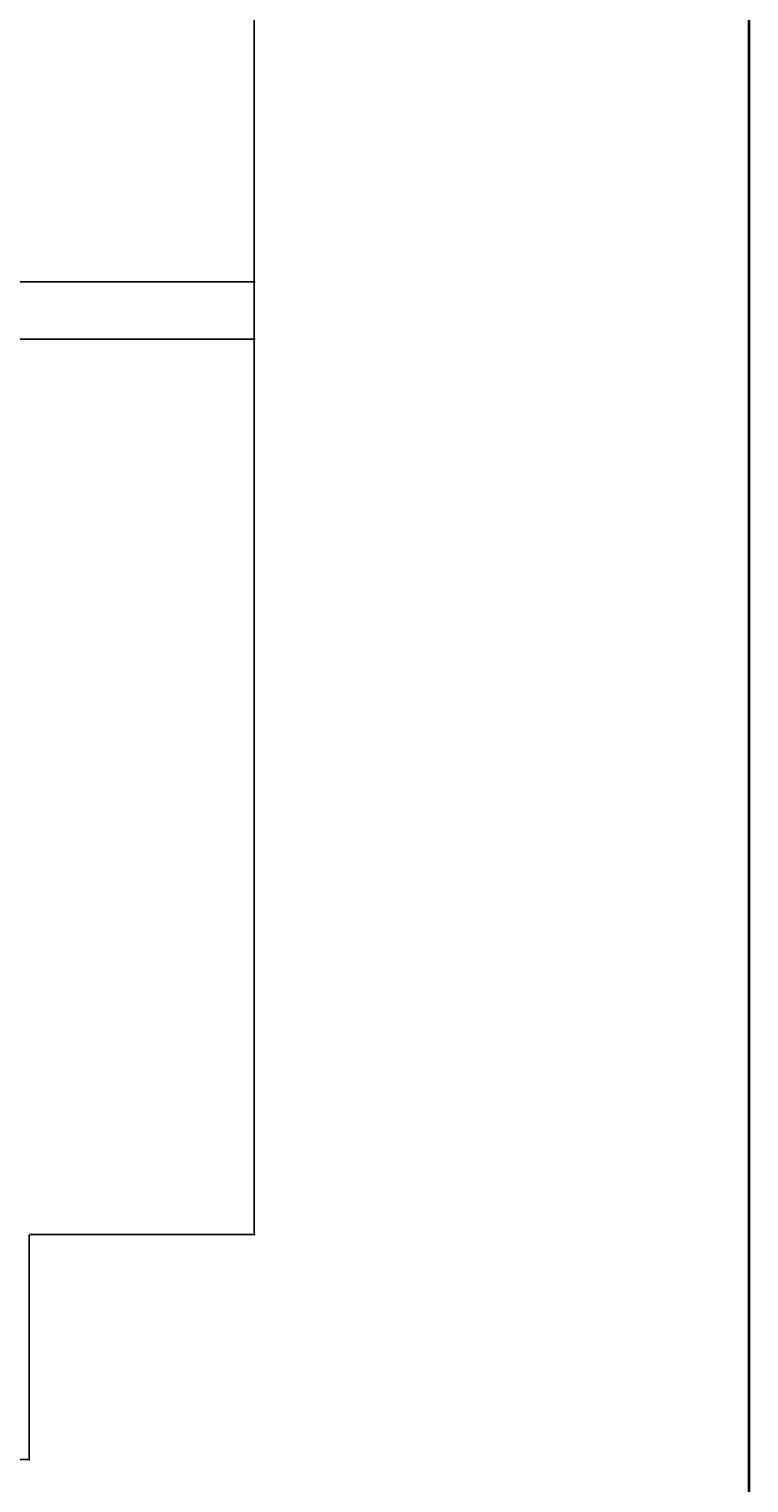
# Model space of a CAD drawing. Units: inches. Extents: x 2234 to 3001, y 1541 to 2386.
# Tile 4 of 12: x 2888 to 3001, y 1663 to 1891. Entities that reach past the tile are written whole.
import ezdxf

# ---------------------------------------------------------------- set-up
doc = ezdxf.new("R2010")
doc.units = ezdxf.units.IN
doc.layers.add('A-ANNO-DIMS', color=2, linetype='Continuous', lineweight=18)
doc.layers.add('A-ANNO-TTLB', color=7, linetype='Continuous', lineweight=35)
doc.styles.get("Standard").update_dxf_attribs({"font": 'arial.ttf'})
doc.dimstyles.get("Standard").update_dxf_attribs({"dimtxt": 0.18, "dimasz": 0.18, "dimexe": 0.18, "dimexo": 0.0625, "dimgap": 0.09, "dimtad": 0, "dimtih": 1, "dimtoh": 1, "dimdec": 4, "dimzin": 0, "dimdsep": 46, "dimtxsty": 'Standard', "dimcen": 0.09, "dimadec": 0, "dimazin": 0, "dimtfac": 1, "dimtdec": 4, "dimtofl": 0, "dimtmove": 0, "dimatfit": 3, "dimfxl": 1, "dimtolj": 1, "dimtzin": 0, "dimarcsym": 0})

# ---------------------------------------------------------------- blocks, each defined once
blk = doc.blocks.new('*D62')
at = {"layer": 'A-ANNO-DIMS', "color": 0, "lineweight": -2, "transparency": 16777216}
for p, q in [((2888.32, 2298.61), (2923.78, 2298.61)), ((2923.6, 2298.43), (2923.6, 2000.54)), ((2923.6, 1702.29), (2923.6, 2000.18)), ((2888.32, 1702.11), (2923.78, 1702.11))]:
    blk.add_line(p, q, dxfattribs=at)
at = {"layer": 'A-ANNO-DIMS', "color": 0, "transparency": 16777216}
for points in [[(2923.57, 2298.43), (2923.63, 2298.43), (2923.6, 2298.61)], [(2923.57, 1702.29), (2923.63, 1702.29), (2923.6, 1702.11)]]:
    blk.add_solid(points, dxfattribs=at)
at = {"layer": 'Defpoints', "color": 0, "transparency": 16777216}
for p in [(2888.25, 2298.61), (2923.6, 2298.61), (2888.25, 1702.11)]:
    blk.add_point(p, dxfattribs=at)
at = {"layer": 'A-ANNO-DIMS', "color": 0, "transparency": 16777216, "insert": (2923.6, 2000.36), "char_height": 0.18, "attachment_point": 5}
blk.add_mtext('\\A1;596.5', dxfattribs=at)
blk = doc.blocks.new('*D66')
at = {"layer": 'A-ANNO-DIMS', "color": 0, "lineweight": -2, "transparency": 16777216}
for p, q in [((2634.82, 1851.65), (2923.78, 1851.65)), ((2923.6, 1851.47), (2923.6, 1847.33)), ((2923.6, 1842.83), (2923.6, 1846.97)), ((2639.32, 1842.65), (2923.78, 1842.65))]:
    blk.add_line(p, q, dxfattribs=at)
at = {"layer": 'A-ANNO-DIMS', "color": 0, "transparency": 16777216}
for points in [[(2923.57, 1851.47), (2923.63, 1851.47), (2923.6, 1851.65)], [(2923.57, 1842.83), (2923.63, 1842.83), (2923.6, 1842.65)]]:
    blk.add_solid(points, dxfattribs=at)
at = {"layer": 'Defpoints', "color": 0, "transparency": 16777216}
for p in [(2634.75, 1851.65), (2923.6, 1851.65), (2639.25, 1842.65)]:
    blk.add_point(p, dxfattribs=at)
at = {"layer": 'A-ANNO-DIMS', "color": 0, "transparency": 16777216, "insert": (2923.6, 1847.15), "char_height": 0.18, "attachment_point": 5}
blk.add_mtext('\\A1;9', dxfattribs=at)
blk = doc.blocks.new('*D74')
at = {"layer": 'A-ANNO-DIMS', "color": 0, "lineweight": -2, "transparency": 16777216}
for p, q in [((2634.75, 1706.55), (2634.75, 1666.58)), ((2888.25, 1702.05), (2888.25, 1666.58)), ((2634.93, 1666.76), (2761.11, 1666.76)), ((2888.07, 1666.76), (2761.9, 1666.76))]:
    blk.add_line(p, q, dxfattribs=at)
at = {"layer": 'A-ANNO-DIMS', "color": 0, "transparency": 16777216}
for points in [[(2634.93, 1666.79), (2634.93, 1666.73), (2634.75, 1666.76)], [(2888.07, 1666.79), (2888.07, 1666.73), (2888.25, 1666.76)]]:
    blk.add_solid(points, dxfattribs=at)
at = {"layer": 'Defpoints', "color": 0, "transparency": 16777216}
for p in [(2634.75, 1706.61), (2888.25, 1702.11), (2888.25, 1666.76)]:
    blk.add_point(p, dxfattribs=at)
at = {"layer": 'A-ANNO-DIMS', "color": 0, "transparency": 16777216, "insert": (2761.5, 1666.76), "char_height": 0.18, "attachment_point": 5}
blk.add_mtext('\\A1;253.5', dxfattribs=at)

msp = doc.modelspace()

# ---------------------------------------------------------------- linework, layer by layer
at = {"layer": 'A-ANNO-TTLB'}
msp.add_lwpolyline([(2233.5367, 2385.7012), (3001.3383, 2385.7012), (3001.3383, 1541.435), (2233.5367, 1541.435)], close=True, dxfattribs=at)

# ---------------------------------------------------------------- dimensions: what is measured, and where the dimension line sits
at = {"layer": 'A-ANNO-DIMS'}
for base, p1, p2, override, picture, middle in [((2923.6034, 2298.611), (2888.2534, 1702.111), (2888.2534, 2298.611), {"dimdec": 1, "dimlfac": 1, "dimrnd": 0, "dimzin": 0, "dimdsep": 46, "dimlunit": 2}, '*D62', (2923.6034, 2000.361)), ((2923.6034, 1851.6488), (2639.2534, 1842.6488), (2634.7534, 1851.6488), {"dimdec": 0, "dimlfac": 1, "dimrnd": 0, "dimzin": 0, "dimdsep": 46, "dimlunit": 2}, '*D66', (2923.6034, 1847.1488))]:
    dim = msp.add_linear_dim(base=base, p1=p1, p2=p2, angle=90, dimstyle='Standard', override=override, dxfattribs=at)
    dim.commit()
    dim.dimension.update_dxf_attribs({"geometry": picture, "text_midpoint": middle})
dim = msp.add_linear_dim(base=(2888.2534, 1666.761), p1=(2634.7534, 1706.611), p2=(2888.2534, 1702.111), dimstyle='Standard', override={"dimdec": 1, "dimlfac": 1, "dimrnd": 0, "dimzin": 0, "dimdsep": 46, "dimlunit": 2}, dxfattribs=at)
dim.commit()
dim.dimension.update_dxf_attribs({"geometry": '*D74', "text_midpoint": (2761.5034, 1666.761)})

doc.saveas('drawing.dxf')
